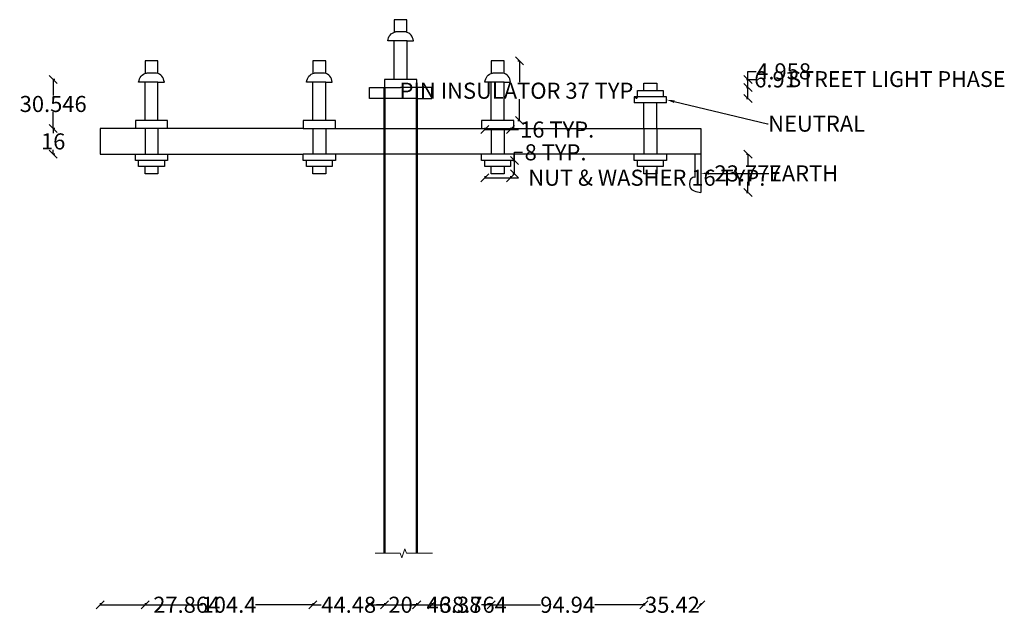
# Model space of a CAD drawing. Units: centimetres. Extents: x -70 to 1009, y -133 to 977.
# Tile 3 of 3: x 397 to 1009, y 396 to 766. Entities that reach past the tile are written whole.
import ezdxf
from ezdxf import colors
from ezdxf.entities.mleader import LeaderData, LeaderLine
from ezdxf.math import Vec2, Vec3

# ---------------------------------------------------------------- set-up
doc = ezdxf.new("R2010")
doc.units = ezdxf.units.CM
doc.header["$MEASUREMENT"] = 0
for name, color, linetype, lineweight in [('E-ANNO-DIMS', 2, 'Continuous', 18), ('E-ANNO-SYMB', 8, 'Continuous', 13), ('E-ANNO-TEXT', 7, 'Continuous', 25), ('E-POLE', 7, 'Continuous', 50), ('E-POLE-HDWR', 4, 'Continuous', 25)]:
    doc.layers.add(name, color=color, linetype=linetype, lineweight=lineweight)
doc.styles.get("Standard").update_dxf_attribs({"font": 'arial.ttf'})
doc.dimstyles.get("Standard").update_dxf_attribs({"dimtxt": 10, "dimasz": 5, "dimexe": 0.1, "dimexo": 0.1, "dimgap": 0.09, "dimtad": 0, "dimtih": 1, "dimtoh": 1, "dimdec": 0, "dimzin": 0, "dimdsep": 46, "dimtxsty": 'Standard', "dimblk": 'OBLIQUE', "dimcen": 0.09, "dimadec": 0, "dimazin": 0, "dimtfac": 1, "dimtdec": 0, "dimtofl": 0, "dimtmove": 0, "dimatfit": 3, "dimfxl": 1, "dimfxlon": 1, "dimtolj": 1, "dimtzin": 0, "dimarcsym": 0})

# ---------------------------------------------------------------- blocks, each defined once
blk = doc.blocks.new('PIN-INSULATOR')
for p, q in [((11.97, 37.12), (4, 37.12)), ((4, 37.12), (4, 29.27)), ((11.97, 29.28), (11.97, 37.12)), ((11.2, 29.48), (4.8, 29.48)), ((4, 23.94), (0, 23.94)), ((4, 0), (4, 23.94)), ((12, 23.94), (4, 23.94)), ((12, 0), (12, 23.94)), ((12, 23.94), (13, 23.94)), ((13, 23.94), (14, 23.94)), ((14, 23.94), (15, 23.94)), ((15, 23.94), (16, 23.94))]:
    blk.add_line(p, q)
for points in [[(0, 23.94), (0.33, 25.27), (0.98, 27.87), (3.53, 29.23), (4.8, 29.48)], [(16, 23.94), (15.67, 25.27), (15.02, 27.87), (12.47, 29.23), (11.2, 29.48)]]:
    blk.add_open_spline(points, degree=3, knots=[0, 0, 0, 0, 3.96368, 7.749621, 7.749621, 7.749621, 7.749621])
blk = doc.blocks.new('NUT-WASHER')
for p, q in [((0, 4.52), (0, 8.38)), ((16.02, 8.38), (16.02, 4.52)), ((16.02, 4.52), (0, 4.52)), ((4, 0), (4, 4.52)), ((12, 0), (4, 0)), ((12, 4.52), (12, 0))]:
    blk.add_line(p, q)
blk = doc.blocks.new('_Oblique')
at = {"color": 0, "linetype": 'ByBlock', "lineweight": -2}
blk.add_line((-0.5, -0.5), (0.5, 0.5), dxfattribs=at)
blk = doc.blocks.new('*D15')
at = {"layer": 'Defpoints', "color": 0, "transparency": 16777216}
for p in [(686.35, 670.6), (702.37, 670.6), (702.37, 668.2)]:
    blk.add_point(p, dxfattribs=at)
at = {"layer": 'E-ANNO-DIMS', "color": 0, "lineweight": -2, "transparency": 16777216}
for p, q in [((686.35, 669.2), (686.35, 668.1)), ((686.35, 668.2), (702.37, 668.2)), ((702.37, 669.2), (702.37, 668.1)), ((702.37, 668.2), (707.37, 668.2))]:
    blk.add_line(p, q, dxfattribs=at)
at = {"layer": 'E-ANNO-DIMS', "color": 0, "lineweight": -2, "transparency": 16777216, "xscale": 5, "yscale": 5, "zscale": 5, "rotation": 180}
blk.add_blockref('_Oblique', (686.35, 668.2), dxfattribs=at)
at = {"layer": 'E-ANNO-DIMS', "color": 0, "lineweight": -2, "transparency": 16777216, "xscale": 5, "yscale": 5, "zscale": 5}
blk.add_blockref('_Oblique', (702.37, 668.2), dxfattribs=at)
at = {"layer": 'E-ANNO-DIMS', "color": 0, "transparency": 16777216, "insert": (787.05, 668.2), "char_height": 10, "attachment_point": 5}
blk.add_mtext('\\A1;NUT & WASHER 16 TYP.', dxfattribs=at)
blk = doc.blocks.new('*D16')
at = {"layer": 'Defpoints', "color": 0, "transparency": 16777216}
for p in [(702.37, 678.99), (704.77, 678.99), (702.37, 670.6)]:
    blk.add_point(p, dxfattribs=at)
at = {"layer": 'E-ANNO-DIMS', "color": 0, "lineweight": -2, "transparency": 16777216}
for p, q in [((704.77, 678.99), (704.77, 683.99)), ((704.77, 683.99), (709.77, 683.99)), ((703.77, 678.99), (704.87, 678.99)), ((704.77, 670.6), (704.77, 678.99)), ((703.77, 670.6), (704.87, 670.6))]:
    blk.add_line(p, q, dxfattribs=at)
at = {"layer": 'E-ANNO-DIMS', "color": 0, "lineweight": -2, "transparency": 16777216, "xscale": 5, "yscale": 5, "zscale": 5}
for p, rotation in [((704.77, 678.99), 90), ((704.77, 670.6), 270)]:
    blk.add_blockref('_Oblique', p, dxfattribs=dict(at, rotation=rotation))
at = {"layer": 'E-ANNO-DIMS', "color": 0, "transparency": 16777216, "insert": (730.32, 683.99), "char_height": 10, "attachment_point": 5}
blk.add_mtext('\\A1;8 TYP.', dxfattribs=at)
blk = doc.blocks.new('*D17')
at = {"layer": 'Defpoints', "color": 0, "transparency": 16777216}
for p in [(702.35, 740.85), (707.91, 740.85), (702.35, 703.73)]:
    blk.add_point(p, dxfattribs=at)
at = {"layer": 'E-ANNO-DIMS', "color": 0, "lineweight": -2, "transparency": 16777216}
for p, q in [((706.91, 740.85), (708.01, 740.85)), ((707.91, 740.85), (707.91, 727.56)), ((707.91, 703.73), (707.91, 717.02)), ((706.91, 703.73), (708.01, 703.73))]:
    blk.add_line(p, q, dxfattribs=at)
at = {"layer": 'E-ANNO-DIMS', "color": 0, "lineweight": -2, "transparency": 16777216, "xscale": 5, "yscale": 5, "zscale": 5}
for p, rotation in [((707.91, 740.85), 90), ((707.91, 703.73), 270)]:
    blk.add_blockref('_Oblique', p, dxfattribs=dict(at, rotation=rotation))
at = {"layer": 'E-ANNO-DIMS', "color": 0, "transparency": 16777216, "insert": (707.91, 722.29), "char_height": 10, "attachment_point": 5}
blk.add_mtext('\\A1;PIN INSULATOR 37 TYP.', dxfattribs=at)
blk = doc.blocks.new('*D18')
at = {"layer": 'Defpoints', "color": 0, "transparency": 16777216}
for p in [(686.35, 703.73), (702.35, 703.73), (702.35, 698.16)]:
    blk.add_point(p, dxfattribs=at)
at = {"layer": 'E-ANNO-DIMS', "color": 0, "lineweight": -2, "transparency": 16777216}
for p, q in [((686.35, 699.16), (686.35, 698.06)), ((686.35, 698.16), (702.35, 698.16)), ((702.35, 699.16), (702.35, 698.06)), ((702.35, 698.16), (707.35, 698.16))]:
    blk.add_line(p, q, dxfattribs=at)
at = {"layer": 'E-ANNO-DIMS', "color": 0, "lineweight": -2, "transparency": 16777216, "xscale": 5, "yscale": 5, "zscale": 5, "rotation": 180}
blk.add_blockref('_Oblique', (686.35, 698.16), dxfattribs=at)
at = {"layer": 'E-ANNO-DIMS', "color": 0, "lineweight": -2, "transparency": 16777216, "xscale": 5, "yscale": 5, "zscale": 5}
blk.add_blockref('_Oblique', (702.35, 698.16), dxfattribs=at)
at = {"layer": 'E-ANNO-DIMS', "color": 0, "transparency": 16777216, "insert": (731.3, 698.16), "char_height": 10, "attachment_point": 5}
blk.add_mtext('\\A1;16 TYP.', dxfattribs=at)
blk = doc.blocks.new('*D37')
at = {"layer": 'Defpoints', "color": 0, "transparency": 16777216}
for p in [(417.98, 698.77), (447.23, 698.77), (447.23, 682.77)]:
    blk.add_point(p, dxfattribs=at)
at = {"layer": 'E-ANNO-DIMS', "color": 0, "lineweight": -2, "transparency": 16777216}
for p, q in [((418.98, 698.77), (417.88, 698.77)), ((417.98, 698.77), (417.98, 695.97)), ((418.98, 682.77), (417.88, 682.77)), ((417.98, 682.77), (417.98, 685.58))]:
    blk.add_line(p, q, dxfattribs=at)
at = {"layer": 'E-ANNO-DIMS', "color": 0, "lineweight": -2, "transparency": 16777216, "xscale": 5, "yscale": 5, "zscale": 5}
for p, rotation in [((417.98, 698.77), 90), ((417.98, 682.77), 270)]:
    blk.add_blockref('_Oblique', p, dxfattribs=dict(at, rotation=rotation))
at = {"layer": 'E-ANNO-DIMS', "color": 0, "transparency": 16777216, "insert": (417.98, 690.77), "char_height": 10, "attachment_point": 5}
blk.add_mtext('\\A1;16', dxfattribs=at)
blk = doc.blocks.new('*D38')
at = {"layer": 'Defpoints', "color": 0, "transparency": 16777216}
for p in [(623.96, 729.32), (417.98, 698.77), (447.23, 698.77)]:
    blk.add_point(p, dxfattribs=at)
at = {"layer": 'E-ANNO-DIMS', "color": 0, "lineweight": -2, "transparency": 16777216}
for p, q in [((418.98, 729.32), (417.88, 729.32)), ((417.98, 729.32), (417.98, 719.25)), ((417.98, 698.77), (417.98, 708.85)), ((418.98, 698.77), (417.88, 698.77))]:
    blk.add_line(p, q, dxfattribs=at)
at = {"layer": 'E-ANNO-DIMS', "color": 0, "lineweight": -2, "transparency": 16777216, "xscale": 5, "yscale": 5, "zscale": 5}
for p, rotation in [((417.98, 729.32), 90), ((417.98, 698.77), 270)]:
    blk.add_blockref('_Oblique', p, dxfattribs=dict(at, rotation=rotation))
at = {"layer": 'E-ANNO-DIMS', "color": 0, "transparency": 16777216, "insert": (417.98, 714.05), "char_height": 10, "attachment_point": 5}
blk.add_mtext('\\A1;30.546', dxfattribs=at)
blk = doc.blocks.new('*D39')
at = {"layer": 'Defpoints', "color": 0, "transparency": 16777216}
for p in [(447.23, 682.77), (475.09, 670.6), (475.09, 402.73)]:
    blk.add_point(p, dxfattribs=at)
at = {"layer": 'E-ANNO-DIMS', "color": 0, "lineweight": -2, "transparency": 16777216}
for p, q in [((447.23, 403.73), (447.23, 402.63)), ((447.23, 402.73), (475.09, 402.73)), ((475.09, 403.73), (475.09, 402.63)), ((475.09, 402.73), (480.09, 402.73))]:
    blk.add_line(p, q, dxfattribs=at)
at = {"layer": 'E-ANNO-DIMS', "color": 0, "lineweight": -2, "transparency": 16777216, "xscale": 5, "yscale": 5, "zscale": 5, "rotation": 180}
blk.add_blockref('_Oblique', (447.23, 402.73), dxfattribs=at)
at = {"layer": 'E-ANNO-DIMS', "color": 0, "lineweight": -2, "transparency": 16777216, "xscale": 5, "yscale": 5, "zscale": 5}
blk.add_blockref('_Oblique', (475.09, 402.73), dxfattribs=at)
at = {"layer": 'E-ANNO-DIMS', "color": 0, "transparency": 16777216, "insert": (501, 402.73), "char_height": 10, "attachment_point": 5}
blk.add_mtext('\\A1;27.864', dxfattribs=at)
blk = doc.blocks.new('*D40')
at = {"layer": 'Defpoints', "color": 0, "transparency": 16777216}
for p in [(475.09, 670.6), (579.48, 670.6), (579.48, 402.73)]:
    blk.add_point(p, dxfattribs=at)
at = {"layer": 'E-ANNO-DIMS', "color": 0, "lineweight": -2, "transparency": 16777216}
for p, q in [((475.09, 403.73), (475.09, 402.63)), ((475.09, 402.73), (510.82, 402.73)), ((579.48, 402.73), (543.76, 402.73)), ((579.48, 403.73), (579.48, 402.63))]:
    blk.add_line(p, q, dxfattribs=at)
at = {"layer": 'E-ANNO-DIMS', "color": 0, "lineweight": -2, "transparency": 16777216, "xscale": 5, "yscale": 5, "zscale": 5, "rotation": 180}
blk.add_blockref('_Oblique', (475.09, 402.73), dxfattribs=at)
at = {"layer": 'E-ANNO-DIMS', "color": 0, "lineweight": -2, "transparency": 16777216, "xscale": 5, "yscale": 5, "zscale": 5}
blk.add_blockref('_Oblique', (579.48, 402.73), dxfattribs=at)
at = {"layer": 'E-ANNO-DIMS', "color": 0, "transparency": 16777216, "insert": (527.29, 402.73), "char_height": 10, "attachment_point": 5}
blk.add_mtext('\\A1;104.4', dxfattribs=at)
blk = doc.blocks.new('*D41')
at = {"layer": 'Defpoints', "color": 0, "transparency": 16777216}
for p in [(579.48, 670.6), (623.96, 434.73), (623.96, 402.73)]:
    blk.add_point(p, dxfattribs=at)
at = {"layer": 'E-ANNO-DIMS', "color": 0, "lineweight": -2, "transparency": 16777216}
for p, q in [((579.48, 403.73), (579.48, 402.63)), ((579.48, 402.73), (584.55, 402.73)), ((623.96, 402.73), (618.9, 402.73)), ((623.96, 403.73), (623.96, 402.63))]:
    blk.add_line(p, q, dxfattribs=at)
at = {"layer": 'E-ANNO-DIMS', "color": 0, "lineweight": -2, "transparency": 16777216, "xscale": 5, "yscale": 5, "zscale": 5, "rotation": 180}
blk.add_blockref('_Oblique', (579.48, 402.73), dxfattribs=at)
at = {"layer": 'E-ANNO-DIMS', "color": 0, "lineweight": -2, "transparency": 16777216, "xscale": 5, "yscale": 5, "zscale": 5}
blk.add_blockref('_Oblique', (623.96, 402.73), dxfattribs=at)
at = {"layer": 'E-ANNO-DIMS', "color": 0, "transparency": 16777216, "insert": (601.72, 402.73), "char_height": 10, "attachment_point": 5}
blk.add_mtext('\\A1;44.48', dxfattribs=at)
blk = doc.blocks.new('*D42')
at = {"layer": 'Defpoints', "color": 0, "transparency": 16777216}
for p in [(623.96, 434.73), (643.96, 434.73), (643.96, 402.73)]:
    blk.add_point(p, dxfattribs=at)
at = {"layer": 'E-ANNO-DIMS', "color": 0, "lineweight": -2, "transparency": 16777216}
for p, q in [((623.96, 403.73), (623.96, 402.63)), ((623.96, 402.73), (626.64, 402.73)), ((643.96, 402.73), (641.28, 402.73)), ((643.96, 403.73), (643.96, 402.63))]:
    blk.add_line(p, q, dxfattribs=at)
at = {"layer": 'E-ANNO-DIMS', "color": 0, "lineweight": -2, "transparency": 16777216, "xscale": 5, "yscale": 5, "zscale": 5, "rotation": 180}
blk.add_blockref('_Oblique', (623.96, 402.73), dxfattribs=at)
at = {"layer": 'E-ANNO-DIMS', "color": 0, "lineweight": -2, "transparency": 16777216, "xscale": 5, "yscale": 5, "zscale": 5}
blk.add_blockref('_Oblique', (643.96, 402.73), dxfattribs=at)
at = {"layer": 'E-ANNO-DIMS', "color": 0, "transparency": 16777216, "insert": (633.96, 402.73), "char_height": 10, "attachment_point": 5}
blk.add_mtext('\\A1;20', dxfattribs=at)
blk = doc.blocks.new('*D43')
at = {"layer": 'Defpoints', "color": 0, "transparency": 16777216}
for p in [(690.35, 670.6), (643.96, 434.73), (690.35, 402.73)]:
    blk.add_point(p, dxfattribs=at)
at = {"layer": 'E-ANNO-DIMS', "color": 0, "lineweight": -2, "transparency": 16777216}
for p, q in [((643.96, 403.73), (643.96, 402.63)), ((643.96, 402.73), (649.98, 402.73)), ((690.35, 402.73), (684.33, 402.73)), ((690.35, 403.73), (690.35, 402.63))]:
    blk.add_line(p, q, dxfattribs=at)
at = {"layer": 'E-ANNO-DIMS', "color": 0, "lineweight": -2, "transparency": 16777216, "xscale": 5, "yscale": 5, "zscale": 5, "rotation": 180}
blk.add_blockref('_Oblique', (643.96, 402.73), dxfattribs=at)
at = {"layer": 'E-ANNO-DIMS', "color": 0, "lineweight": -2, "transparency": 16777216, "xscale": 5, "yscale": 5, "zscale": 5}
blk.add_blockref('_Oblique', (690.35, 402.73), dxfattribs=at)
at = {"layer": 'E-ANNO-DIMS', "color": 0, "transparency": 16777216, "insert": (667.16, 402.73), "char_height": 10, "attachment_point": 5}
blk.add_mtext('\\A1;46.38', dxfattribs=at)
blk = doc.blocks.new('*D44')
at = {"layer": 'Defpoints', "color": 0, "transparency": 16777216}
for p in [(690.35, 670.6), (785.28, 670.6), (785.28, 402.73)]:
    blk.add_point(p, dxfattribs=at)
at = {"layer": 'E-ANNO-DIMS', "color": 0, "lineweight": -2, "transparency": 16777216}
for p, q in [((690.35, 403.73), (690.35, 402.63)), ((690.35, 402.73), (720.87, 402.73)), ((785.28, 402.73), (754.76, 402.73)), ((785.28, 403.73), (785.28, 402.63))]:
    blk.add_line(p, q, dxfattribs=at)
at = {"layer": 'E-ANNO-DIMS', "color": 0, "lineweight": -2, "transparency": 16777216, "xscale": 5, "yscale": 5, "zscale": 5, "rotation": 180}
blk.add_blockref('_Oblique', (690.35, 402.73), dxfattribs=at)
at = {"layer": 'E-ANNO-DIMS', "color": 0, "lineweight": -2, "transparency": 16777216, "xscale": 5, "yscale": 5, "zscale": 5}
blk.add_blockref('_Oblique', (785.28, 402.73), dxfattribs=at)
at = {"layer": 'E-ANNO-DIMS', "color": 0, "transparency": 16777216, "insert": (737.82, 402.73), "char_height": 10, "attachment_point": 5}
blk.add_mtext('\\A1;94.94', dxfattribs=at)
blk = doc.blocks.new('*D45')
at = {"layer": 'Defpoints', "color": 0, "transparency": 16777216}
for p in [(820.7, 682.77), (785.28, 670.6), (820.7, 402.73)]:
    blk.add_point(p, dxfattribs=at)
at = {"layer": 'E-ANNO-DIMS', "color": 0, "lineweight": -2, "transparency": 16777216}
for p, q in [((785.28, 403.73), (785.28, 402.63)), ((785.28, 402.73), (786.08, 402.73)), ((820.7, 402.73), (819.9, 402.73)), ((820.7, 403.73), (820.7, 402.63))]:
    blk.add_line(p, q, dxfattribs=at)
at = {"layer": 'E-ANNO-DIMS', "color": 0, "lineweight": -2, "transparency": 16777216, "xscale": 5, "yscale": 5, "zscale": 5, "rotation": 180}
blk.add_blockref('_Oblique', (785.28, 402.73), dxfattribs=at)
at = {"layer": 'E-ANNO-DIMS', "color": 0, "lineweight": -2, "transparency": 16777216, "xscale": 5, "yscale": 5, "zscale": 5}
blk.add_blockref('_Oblique', (820.7, 402.73), dxfattribs=at)
at = {"layer": 'E-ANNO-DIMS', "color": 0, "transparency": 16777216, "insert": (802.99, 402.73), "char_height": 10, "attachment_point": 5}
blk.add_mtext('\\A1;35.42', dxfattribs=at)
blk = doc.blocks.new('*D46')
at = {"layer": 'Defpoints', "color": 0, "transparency": 16777216}
for p in [(820.7, 682.77), (820.7, 659), (849.95, 659)]:
    blk.add_point(p, dxfattribs=at)
at = {"layer": 'E-ANNO-DIMS', "color": 0, "lineweight": -2, "transparency": 16777216}
for p, q in [((848.95, 682.77), (850.05, 682.77)), ((849.95, 682.77), (849.95, 676.08)), ((849.95, 659), (849.95, 665.69)), ((848.95, 659), (850.05, 659))]:
    blk.add_line(p, q, dxfattribs=at)
at = {"layer": 'E-ANNO-DIMS', "color": 0, "lineweight": -2, "transparency": 16777216, "xscale": 5, "yscale": 5, "zscale": 5}
for p, rotation in [((849.95, 682.77), 90), ((849.95, 659), 270)]:
    blk.add_blockref('_Oblique', p, dxfattribs=dict(at, rotation=rotation))
at = {"layer": 'E-ANNO-DIMS', "color": 0, "transparency": 16777216, "insert": (849.95, 670.88), "char_height": 10, "attachment_point": 5}
blk.add_mtext('\\A1;23.777', dxfattribs=at)
blk = doc.blocks.new('*D47')
at = {"layer": 'Defpoints', "color": 0, "transparency": 16777216}
for p in [(614.58, 717.45), (653.35, 717.45), (653.35, 402.73)]:
    blk.add_point(p, dxfattribs=at)
at = {"layer": 'E-ANNO-DIMS', "color": 0, "lineweight": -2, "transparency": 16777216}
for p, q in [((614.58, 403.73), (614.58, 402.63)), ((614.58, 402.73), (653.35, 402.73)), ((653.35, 403.73), (653.35, 402.63)), ((653.35, 402.73), (658.35, 402.73))]:
    blk.add_line(p, q, dxfattribs=at)
at = {"layer": 'E-ANNO-DIMS', "color": 0, "lineweight": -2, "transparency": 16777216, "xscale": 5, "yscale": 5, "zscale": 5, "rotation": 180}
blk.add_blockref('_Oblique', (614.58, 402.73), dxfattribs=at)
at = {"layer": 'E-ANNO-DIMS', "color": 0, "lineweight": -2, "transparency": 16777216, "xscale": 5, "yscale": 5, "zscale": 5}
blk.add_blockref('_Oblique', (653.35, 402.73), dxfattribs=at)
at = {"layer": 'E-ANNO-DIMS', "color": 0, "transparency": 16777216, "insert": (679.17, 402.73), "char_height": 10, "attachment_point": 5}
blk.add_mtext('\\A1;38.764', dxfattribs=at)
blk = doc.blocks.new('*D48')
at = {"layer": 'Defpoints', "color": 0, "transparency": 16777216}
for p in [(653.35, 724.36), (849.95, 724.36), (653.35, 717.45)]:
    blk.add_point(p, dxfattribs=at)
at = {"layer": 'E-ANNO-DIMS', "color": 0, "lineweight": -2, "transparency": 16777216}
for p, q in [((849.95, 724.36), (849.95, 729.36)), ((849.95, 729.36), (854.95, 729.36)), ((848.95, 724.36), (850.05, 724.36)), ((849.95, 717.45), (849.95, 724.36)), ((848.95, 717.45), (850.05, 717.45))]:
    blk.add_line(p, q, dxfattribs=at)
at = {"layer": 'E-ANNO-DIMS', "color": 0, "lineweight": -2, "transparency": 16777216, "xscale": 5, "yscale": 5, "zscale": 5}
for p, rotation in [((849.95, 724.36), 90), ((849.95, 717.45), 270)]:
    blk.add_blockref('_Oblique', p, dxfattribs=dict(at, rotation=rotation))
at = {"layer": 'E-ANNO-DIMS', "color": 0, "transparency": 16777216, "insert": (867.09, 729.36), "char_height": 10, "attachment_point": 5}
blk.add_mtext('\\A1;6.91', dxfattribs=at)
blk = doc.blocks.new('*D49')
at = {"layer": 'Defpoints', "color": 0, "transparency": 16777216}
for p in [(643.96, 729.32), (849.95, 729.32), (643.96, 724.36)]:
    blk.add_point(p, dxfattribs=at)
at = {"layer": 'E-ANNO-DIMS', "color": 0, "lineweight": -2, "transparency": 16777216}
for p, q in [((848.95, 729.32), (850.05, 729.32)), ((849.95, 729.32), (849.95, 734.32)), ((849.95, 734.32), (854.95, 734.32)), ((849.95, 724.36), (849.95, 729.32)), ((848.95, 724.36), (850.05, 724.36))]:
    blk.add_line(p, q, dxfattribs=at)
at = {"layer": 'E-ANNO-DIMS', "color": 0, "lineweight": -2, "transparency": 16777216, "xscale": 5, "yscale": 5, "zscale": 5}
for p, rotation in [((849.95, 729.32), 90), ((849.95, 724.36), 270)]:
    blk.add_blockref('_Oblique', p, dxfattribs=dict(at, rotation=rotation))
at = {"layer": 'E-ANNO-DIMS', "color": 0, "transparency": 16777216, "insert": (872.12, 734.32), "char_height": 10, "attachment_point": 5}
blk.add_mtext('\\A1;4.958', dxfattribs=at)

msp = doc.modelspace()

# ---------------------------------------------------------------- linework, layer by layer
at = {"layer": 'E-ANNO-SYMB'}
msp.add_lwpolyline([(618.1847, 434.7283), (633.6778, 434.7283), (634.6778, 431.9808), (636.6778, 437.4758), (637.6778, 434.7283), (653.8455, 434.7283)], dxfattribs=at)
at = {"layer": 'E-POLE'}
for p, q in [((623.9644, 724.3613), (623.9644, 434.7283)), ((643.9644, 724.3613), (643.9644, 434.7283))]:
    msp.add_line(p, q, dxfattribs=at)
at = {"layer": 'E-POLE-HDWR'}
for p, q in [((643.9644, 729.3194), (623.9644, 729.3194)), ((623.9644, 729.3194), (623.9644, 724.3613)), ((643.9644, 724.3613), (643.9644, 729.3194)), ((614.5823, 717.4515), (614.5823, 724.3613)), ((614.5823, 724.3613), (633.9644, 724.3613)), ((653.3464, 724.3613), (633.9644, 724.3613)), ((653.3464, 717.4515), (653.3464, 724.3613)), ((623.9644, 717.4515), (614.5823, 717.4515)), ((643.9644, 717.4515), (623.9644, 717.4515)), ((643.9644, 717.4515), (653.3464, 717.4515)), ((799.2836, 718.5585), (779.2836, 718.5585)), ((779.2836, 718.5585), (779.2836, 714.7729)), ((799.2836, 714.7729), (799.2836, 718.5585)), ((799.2836, 714.7729), (779.2836, 714.7729)), ((785.2836, 698.7729), (785.2836, 714.7729)), ((793.2836, 698.7729), (793.2836, 714.7729)), ((573.4644, 698.7729), (447.2285, 698.7729)), ((447.2285, 698.7729), (447.2285, 682.7729)), ((489.0924, 703.731), (469.0924, 703.731)), ((469.0924, 703.731), (469.0924, 698.7729)), ((475.0924, 698.7729), (475.0924, 682.7729)), ((483.0924, 698.7729), (483.0924, 682.7729)), ((489.0924, 698.7729), (489.0924, 703.731)), ((573.4644, 698.7729), (694.4644, 698.7729)), ((593.4824, 703.731), (573.4824, 703.731)), ((573.4824, 703.731), (573.4824, 698.7729)), ((579.4824, 698.7729), (579.4824, 682.7729)), ((587.4824, 698.7729), (587.4824, 682.7729)), ((593.4824, 698.7729), (593.4824, 703.731)), ((704.3465, 703.731), (684.3465, 703.731)), ((684.3465, 703.731), (684.3465, 698.7729)), ((690.3465, 698.7729), (690.3465, 682.7729)), ((694.4644, 698.7729), (820.7002, 698.7729)), ((698.3465, 698.7729), (698.3465, 682.7729)), ((704.3465, 698.7729), (704.3465, 703.731)), ((785.2836, 698.7729), (785.2836, 682.7729)), ((793.2836, 698.7729), (793.2836, 682.7729)), ((820.7002, 698.7729), (820.7002, 682.7729)), ((447.2285, 682.7729), (573.4644, 682.7729)), ((469.0924, 678.9874), (469.0924, 682.7729)), ((489.0924, 682.7729), (489.0924, 678.9874)), ((694.4644, 682.7729), (573.4644, 682.7729)), ((573.4824, 678.9874), (573.4824, 682.7729)), ((593.4824, 682.7729), (593.4824, 678.9874)), ((684.3465, 678.9874), (684.3465, 682.7729)), ((820.7002, 682.7729), (694.4644, 682.7729)), ((704.3465, 682.7729), (704.3465, 678.9874)), ((779.2836, 678.9874), (779.2836, 682.7729)), ((799.2836, 682.7729), (799.2836, 678.9874)), ((816.9838, 682.7729), (816.9838, 668.3903)), ((820.7002, 682.7729), (820.7002, 658.9955)), ((489.0924, 678.9874), (469.0924, 678.9874)), ((593.4824, 678.9874), (573.4824, 678.9874)), ((704.3465, 678.9874), (684.3465, 678.9874)), ((799.2836, 678.9874), (779.2836, 678.9874))]:
    msp.add_line(p, q, dxfattribs=at)
msp.add_open_spline([(816.9838, 668.3903), (816.5063, 668.4394), (813.8955, 668.7078), (812.4004, 660.3297), (817.7317, 659.4727), (820.7002, 658.9955)], degree=3, knots=[0, 0, 0, 0, 1.36985271, 7.48967384, 15.17826428, 15.17826428, 15.17826428, 15.17826428], dxfattribs=at)

# ---------------------------------------------------------------- block references
for name, p in [('PIN-INSULATOR', (625.964, 729.319)), ('PIN-INSULATOR', (471.0921, 703.7306)), ('PIN-INSULATOR', (575.482, 703.7306)), ('PIN-INSULATOR', (686.3461, 703.7306)), ('NUT-WASHER', (471.092, 670.604)), ('NUT-WASHER', (575.4819, 670.604)), ('NUT-WASHER', (686.346, 670.604)), ('NUT-WASHER', (781.2831, 670.604))]:
    msp.add_blockref(name, p, dxfattribs=at)
at = {"layer": 'E-POLE-HDWR', "rotation": 180.0308630079717}
msp.add_blockref('NUT-WASHER', (797.292, 726.9462), dxfattribs=at)

# ---------------------------------------------------------------- texts
at = {"layer": 'E-ANNO-TEXT', "insert": (875.0515, 734.4429), "char_height": 9.835469, "attachment_point": 1}
msp.add_mtext_dynamic_manual_height_columns('STREET LIGHT PHASE', width=351.223506, gutter_width=1.9671, heights=[0], dxfattribs=at)

# ---------------------------------------------------------------- dimensions: what is measured, and where the dimension line sits
at = {"layer": 'E-ANNO-DIMS'}
for base, p1, p2, text, picture, middle in [((707.9146, 740.8515), (702.3465, 703.731), (702.3465, 740.8515), 'PIN INSULATOR <> TYP.', '*D17', (707.9146, 722.2912)), ((704.7692, 678.9874), (702.3662, 670.6042), (702.3662, 678.9874), '<> TYP.', '*D16', (730.3196, 683.9874))]:
    dim = msp.add_linear_dim(base=base, p1=p1, p2=p2, angle=90, text=text, dimstyle='Standard', override={"dimdec": 0, "dimrnd": 0, "dimzin": 0, "dimlunit": 2}, dxfattribs=at)
    dim.commit()
    dim.dimension.update_dxf_attribs({"geometry": picture, "text_midpoint": middle})
for base, p1, p2, override, picture, middle in [((849.9502, 729.3194), (643.9644, 724.3613), (643.9644, 729.3194), {"dimdec": 3, "dimlfac": 1, "dimrnd": 0, "dimzin": 0, "dimdsep": 46, "dimlunit": 2}, '*D49', (872.1241, 734.3194)), ((849.9502, 724.3613), (653.3464, 717.4515), (653.3464, 724.3613), {"dimdec": 2, "dimlfac": 1, "dimrnd": 0, "dimzin": 0, "dimdsep": 46, "dimlunit": 2}, '*D48', (867.09, 729.3613)), ((417.97854, 698.77294), (623.96436, 729.31941), (447.22854, 698.77294), {"dimdec": 3, "dimlfac": 1, "dimrnd": 0, "dimzin": 0, "dimdsep": 46, "dimlunit": 2}, '*D38', (417.97854, 714.04617)), ((417.9785, 698.7729), (447.2285, 682.7729), (447.2285, 698.7729), {"dimdec": 0, "dimlfac": 1, "dimrnd": 0, "dimzin": 0, "dimdsep": 46, "dimlunit": 2}, '*D37', (417.9785, 690.7729)), ((849.9502, 658.9955), (820.7002, 682.7729), (820.7002, 658.9955), {"dimdec": 3, "dimlfac": 1, "dimrnd": 0, "dimzin": 0, "dimdsep": 46, "dimlunit": 2}, '*D46', (849.9502, 670.8842))]:
    dim = msp.add_linear_dim(base=base, p1=p1, p2=p2, angle=90, dimstyle='Standard', override=override, dxfattribs=at)
    dim.commit()
    dim.dimension.update_dxf_attribs({"geometry": picture, "text_midpoint": middle})
for base, p1, p2, override, picture, middle in [((653.3464, 402.7308), (614.5823, 717.4515), (653.3464, 717.4515), {"dimdec": 3, "dimlfac": 1, "dimrnd": 0, "dimzin": 0, "dimdsep": 46, "dimlunit": 2}, '*D47', (679.1697, 402.7308)), ((475.0924, 402.7308), (447.2285, 682.7729), (475.0924, 670.6042), {"dimdec": 3, "dimlfac": 1, "dimrnd": 0, "dimzin": 0, "dimdsep": 46, "dimlunit": 2}, '*D39', (501.0044, 402.7308)), ((820.7002, 402.7308), (785.2836, 670.6042), (820.7002, 682.7729), {"dimdec": 2, "dimlfac": 1, "dimrnd": 0, "dimzin": 0, "dimdsep": 46, "dimlunit": 2}, '*D45', (802.9919, 402.7308)), ((579.4824, 402.7308), (475.0924, 670.6042), (579.4824, 670.6042), {"dimdec": 1, "dimlfac": 1, "dimrnd": 0, "dimzin": 0, "dimdsep": 46, "dimlunit": 2}, '*D40', (527.2874, 402.7308)), ((623.9644, 402.7308), (579.4824, 670.6042), (623.9644, 434.7283), {"dimdec": 2, "dimlfac": 1, "dimrnd": 0, "dimzin": 0, "dimdsep": 46, "dimlunit": 2}, '*D41', (601.7234, 402.7308)), ((690.3465, 402.7308), (643.9644, 434.7283), (690.3465, 670.6042), {"dimdec": 2, "dimlfac": 1, "dimrnd": 0, "dimzin": 0, "dimdsep": 46, "dimlunit": 2}, '*D43', (667.1554, 402.7308)), ((785.2836, 402.7308), (690.3465, 670.6042), (785.2836, 670.6042), {"dimdec": 2, "dimlfac": 1, "dimrnd": 0, "dimzin": 0, "dimdsep": 46, "dimlunit": 2}, '*D44', (737.815, 402.7308)), ((643.9644, 402.7308), (623.9644, 434.7283), (643.9644, 434.7283), {"dimdec": 0, "dimlfac": 1, "dimrnd": 0, "dimzin": 0, "dimdsep": 46, "dimlunit": 2}, '*D42', (633.9644, 402.7308))]:
    dim = msp.add_linear_dim(base=base, p1=p1, p2=p2, dimstyle='Standard', override=override, dxfattribs=at)
    dim.commit()
    dim.dimension.update_dxf_attribs({"geometry": picture, "text_midpoint": middle})
for base, p1, p2, text, picture, middle in [((702.3465, 698.1629), (686.3465, 703.731), (702.3465, 703.731), '<> TYP.', '*D18', (731.3042, 698.1629)), ((702.3662, 668.2012), (686.3465, 670.6042), (702.3662, 670.6042), 'NUT & WASHER <> TYP.', '*D15', (787.0469, 668.2012))]:
    dim = msp.add_linear_dim(base=base, p1=p1, p2=p2, text=text, dimstyle='Standard', override={"dimdec": 0, "dimrnd": 0, "dimzin": 0, "dimlunit": 2}, dxfattribs=at)
    dim.commit()
    dim.dimension.update_dxf_attribs({"geometry": picture, "text_midpoint": middle})

# ---------------------------------------------------------------- leaders
at = {"layer": 'E-ANNO-TEXT'}
ml = msp.add_multileader_mtext('Standard', dxfattribs=at)
ml.set_content('NEUTRAL', color=256)
ml.set_leader_properties()
ml.build(insert=Vec2(0, 0))
ml.multileader.update_dxf_attribs({"dogleg_length": 0.36, "arrow_head_size": 5})
ctx = ml.context
ctx.base_point, ctx.char_height, ctx.arrow_head_size, ctx.landing_gap_size, ctx.plane_origin = Vec3(862.4143, 701.7368), 10, 5, 0.09, Vec3(799.2836, 716.6657)
notes = []
notes.append((ctx, [(0, (1, 1, 0), (862.0543, 701.7368), (1, 0), 0.36, [(0, [(799.2836, 716.6657)], 0, [])])]))
ctx.mtext.insert, ctx.mtext.flow_direction = Vec3(862.5043, 706.8221), 5
ml = msp.add_multileader_mtext('Standard', dxfattribs=at)
ml.set_content('EARTH', color=256)
ml.set_leader_properties()
ml.build(insert=Vec2(0, 0))
ml.multileader.update_dxf_attribs({"dogleg_length": 0.36, "arrow_head_size": 5})
ctx = ml.context
ctx.base_point, ctx.char_height, ctx.arrow_head_size, ctx.landing_gap_size, ctx.plane_origin = Vec3(862.8643, 670.8842), 10, 5, 0.09, Vec3(820.7002, 670.8842)
notes.append((ctx, [(0, (1, 1, 0), (862.5043, 670.8842), (1, 0), 0.36, [(0, [(820.7002, 670.8842)], 0, [])])]))
ctx.mtext.insert, ctx.mtext.flow_direction = Vec3(862.9543, 675.8842), 5
for ctx, leaders in notes:
    for number, flags, end, landing, length, lines in leaders:
        leader = LeaderData()
        leader.index, (leader.has_last_leader_line, leader.has_dogleg_vector, leader.attachment_direction) = number, flags
        leader.last_leader_point, leader.dogleg_vector, leader.dogleg_length = Vec3(end), Vec3(landing), length
        for number, points, colour, breaks in lines:
            line = LeaderLine()
            line.index, line.vertices, line.color, line.breaks = number, Vec3.list(points), colors.encode_raw_color(colour), breaks
            leader.lines.append(line)
        ctx.leaders.append(leader)

doc.saveas('drawing.dxf')
